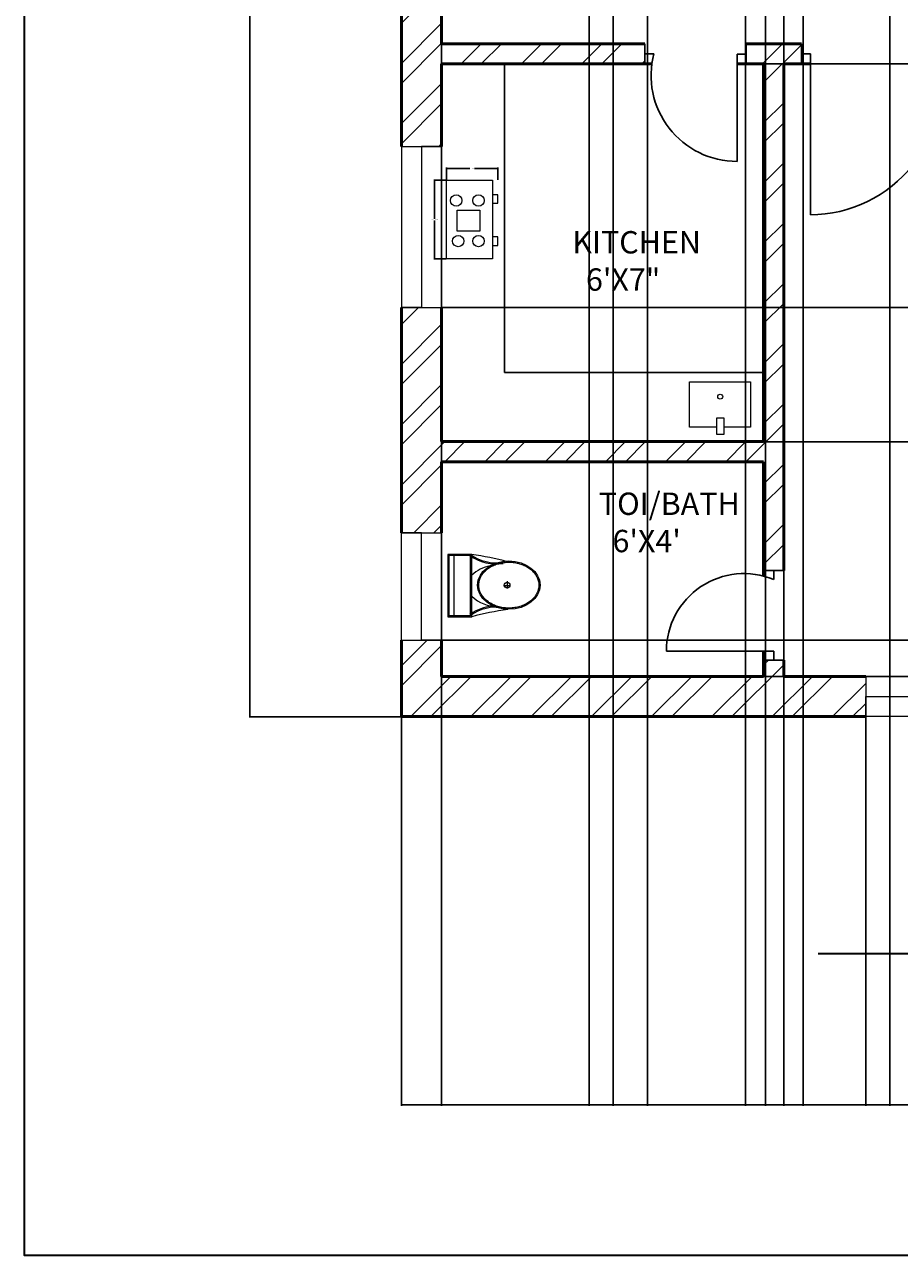
# Model space of a CAD drawing. Units: inches. Extents: x 2310 to 2937, y 1113 to 2410.
# Tile 1 of 23: x 2310 to 2506, y 1616 to 1891. Entities that reach past the tile are written whole.
import ezdxf

# ---------------------------------------------------------------- set-up
doc = ezdxf.new("R2010")
doc.units = ezdxf.units.IN
for name, color, linetype, lineweight in [('A-ANNO-DIMS', 2, 'Continuous', 18), ('A-ANNO-TTLB', 7, 'Continuous', 35), ('A-AREA-IDEN', 7, 'Continuous', 18), ('A-DOOR', 31, 'Continuous', 25), ('A-EQPM', 8, 'Continuous', 18), ('A-FLOR-CASE', 7, 'Continuous', 25), ('A-FLOR-FIXT', 9, 'Continuous', 18), ('A-GLAZ', 191, 'Continuous', 20), ('A-WALL', 7, 'Continuous', 50), ('A-WALL-PATT', 85, 'Continuous', 13)]:
    doc.layers.add(name, color=color, linetype=linetype, lineweight=lineweight)
doc.styles.get("Standard").update_dxf_attribs({"font": 'arial.ttf'})
doc.dimstyles.get("Standard").update_dxf_attribs({"dimtxt": 0.18, "dimasz": 0.18, "dimexe": 0.18, "dimexo": 0.0625, "dimgap": 0.09, "dimtad": 0, "dimtih": 1, "dimtoh": 1, "dimdec": 4, "dimzin": 0, "dimdsep": 46, "dimtxsty": 'Standard', "dimcen": 0.09, "dimadec": 0, "dimazin": 0, "dimtfac": 1, "dimtdec": 4, "dimtofl": 0, "dimtmove": 0, "dimatfit": 3, "dimfxl": 1, "dimtolj": 1, "dimtzin": 0, "dimarcsym": 0})

# ---------------------------------------------------------------- blocks, each defined once
blk = doc.blocks.new('A$C31115884')
for p, q in [((258, 466), (258, 523)), ((283, 498), (223, 498)), ((0, 200), (0, 0)), ((520, 200), (0, 200)), ((10, 190), (10, 10)), ((510, 190), (10, 190)), ((510, 10), (510, 190)), ((520, 0), (520, 200)), ((510, 54), (0, 54)), ((10, 10), (510, 10)), ((0, 0), (520, 0))]:
    blk.add_line(p, q)
blk.add_circle((256, 496), 23.6)
for centre, radius, start, end in [((2778, -205), 2807, 165.4549, 171.7133), ((-295, 403), 365, 324.2091, 9.3499), ((-295, 403), 375, 324.2091, 9.3499), ((139, 406), 293, 315.8436, 2.6563), ((806, 403), 365, 170.6501, 215.7909), ((3237, 905), 2807, 188.2867, 194.5451), ((384, 406), 293, 190.2774, 224.1564), ((806, 403), 375, 179.2036, 215.7909)]:
    blk.add_arc(centre, radius, start, end)
blk.add_ellipse((256, 510), major_axis=(0, -261), ratio=0.772727)
blk.add_open_spline([(256, 259), (263, 259), (270, 260), (288, 262), (299, 265), (320, 273), (330, 278), (350, 291), (360, 299), (378, 316), (386, 326), (402, 347), (409, 358), (421, 383), (427, 395), (436, 422), (440, 436), (445, 465), (447, 480), (448, 509), (448, 524), (445, 553), (443, 568), (436, 596), (432, 610), (422, 636), (416, 649), (402, 672), (395, 683), (379, 703), (370, 712), (351, 728), (341, 735), (321, 746), (310, 751), (289, 757), (278, 759), (256, 761), (245, 761), (223, 757), (212, 754), (191, 746), (181, 741), (161, 728), (151, 720), (133, 703), (125, 693), (110, 672), (103, 660), (90, 636), (85, 623), (76, 596), (72, 582), (67, 553), (66, 538), (64, 509), (65, 494), (68, 465), (70, 450), (77, 422), (81, 408), (91, 382), (97, 370), (111, 346), (118, 335), (135, 316), (144, 307), (162, 291), (172, 284), (193, 273), (203, 269), (225, 262), (236, 260), (250, 259), (253, 259), (256, 259)], degree=3, knots=[0, 0, 0, 0, 0.110105, 0.110105, 0.285049, 0.285049, 0.459994, 0.459994, 0.634938, 0.634938, 0.809882, 0.809882, 0.984827, 0.984827, 1.159771, 1.159771, 1.334715, 1.334715, 1.50966, 1.50966, 1.684604, 1.684604, 1.859549, 1.859549, 2.034493, 2.034493, 2.209437, 2.209437, 2.384382, 2.384382, 2.559326, 2.559326, 2.73427, 2.73427, 2.909215, 2.909215, 3.084159, 3.084159, 3.259103, 3.259103, 3.434048, 3.434048, 3.608992, 3.608992, 3.783936, 3.783936, 3.958881, 3.958881, 4.133825, 4.133825, 4.30877, 4.30877, 4.483714, 4.483714, 4.658658, 4.658658, 4.833603, 4.833603, 5.008547, 5.008547, 5.183491, 5.183491, 5.358436, 5.358436, 5.53338, 5.53338, 5.708324, 5.708324, 5.883269, 5.883269, 6.058213, 6.058213, 6.233158, 6.233158, 6.283185, 6.283185, 6.283185, 6.283185])
blk = doc.blocks.new('SINK-KITCHEN')
blk.add_lwpolyline([(6.01, 11.79), (7.56, 11.79), (7.56, 8.11), (6.01, 8.11)], close=True)
blk.add_lwpolyline([(7.56, 10.17), (13.64, 10.17), (13.64, 0), (0, 0), (0, 10.17), (6.01, 10.17)])
blk.add_circle((6.79, 3.34), 0.556)
blk = doc.blocks.new('RANGE-4-BURNER')
for points in [[(1.2, 17.61), (1.2, 17.61), (1.2, 17.61), (1.2, 17.61)], [(1.2, 17.61), (11.5, 17.61), (11.5, 0), (1.2, 0)], [(1.2, 14.58), (0, 14.58), (0, 12.67), (1.2, 12.67)], [(4.01, 11.43), (9.13, 11.43), (9.13, 6.73), (4.01, 6.73)], [(1.2, 5.14), (0, 5.14), (0, 3.24), (1.2, 3.24)]]:
    blk.add_lwpolyline(points, close=True)
for centre in [(4.34, 13.6), (8.87, 13.6), (4.34, 4.53), (9.32, 4.53)]:
    blk.add_circle(centre, 1.27)
blk = doc.blocks.new('WIN-24IN')
for p, q in [((0, 24), (9, 24)), ((0, 24), (0, 0)), ((9, 24), (4.5, 24)), ((4.5, 24), (4.5, 0)), ((9, 24), (9, 0)), ((4.5, 0), (0, 0)), ((0, 0), (9, 0))]:
    blk.add_line(p, q)
blk = doc.blocks.new('WIN-60IN')
for p, q in [((4.5, 60), (0, 60)), ((0, 60), (9, 60)), ((0, 60), (0, 0)), ((4.5, 0), (4.5, 60)), ((9, 60), (9, 0)), ((0, 0), (9, 0)), ((9, 0), (4.5, 0))]:
    blk.add_line(p, q)
blk = doc.blocks.new('*D25')
at = {"layer": 'A-ANNO-DIMS', "color": 0, "lineweight": -2, "transparency": 16777216}
for p, q in [((2404.5, 1856.48), (2401.74, 1856.48)), ((2401.92, 1856.3), (2401.92, 1847.86)), ((2401.92, 1839.05), (2401.92, 1847.49)), ((2404.5, 1838.87), (2401.74, 1838.87))]:
    blk.add_line(p, q, dxfattribs=at)
at = {"layer": 'A-ANNO-DIMS', "color": 0, "transparency": 16777216}
for points in [[(2401.89, 1856.3), (2401.95, 1856.3), (2401.92, 1856.48)], [(2401.89, 1839.05), (2401.95, 1839.05), (2401.92, 1838.87)]]:
    blk.add_solid(points, dxfattribs=at)
at = {"layer": 'Defpoints', "color": 0, "transparency": 16777216}
for p in [(2404.57, 1856.48), (2401.92, 1838.87), (2404.57, 1838.87)]:
    blk.add_point(p, dxfattribs=at)
at = {"layer": 'A-ANNO-DIMS', "color": 0, "transparency": 16777216, "insert": (2401.92, 1847.67), "char_height": 0.18, "attachment_point": 5}
blk.add_mtext('\\A1;RANGE 18 TYP.', dxfattribs=at)
blk = doc.blocks.new('*D26')
at = {"layer": 'A-ANNO-DIMS', "color": 0, "lineweight": -2, "transparency": 16777216}
for p, q in [((2404.57, 1856.54), (2404.57, 1859.3)), ((2404.75, 1859.12), (2409.8, 1859.12)), ((2415.89, 1859.12), (2410.84, 1859.12)), ((2416.07, 1856.54), (2416.07, 1859.3))]:
    blk.add_line(p, q, dxfattribs=at)
at = {"layer": 'A-ANNO-DIMS', "color": 0, "transparency": 16777216}
for points in [[(2404.75, 1859.15), (2404.75, 1859.09), (2404.57, 1859.12)], [(2415.89, 1859.15), (2415.89, 1859.09), (2416.07, 1859.12)]]:
    blk.add_solid(points, dxfattribs=at)
at = {"layer": 'Defpoints', "color": 0, "transparency": 16777216}
for p in [(2404.57, 1859.12), (2404.57, 1856.48), (2416.07, 1856.48)]:
    blk.add_point(p, dxfattribs=at)
at = {"layer": 'A-ANNO-DIMS', "color": 0, "transparency": 16777216, "insert": (2410.32, 1859.12), "char_height": 0.18, "attachment_point": 5}
blk.add_mtext('\\A1;12 TYP.', dxfattribs=at)
blk = doc.blocks.new('*D40')
at = {"layer": 'A-ANNO-DIMS', "color": 0, "lineweight": -2, "transparency": 16777216}
for p, q in [((2394.42, 2356.51), (2360.46, 2356.51)), ((2360.64, 2356.33), (2360.64, 2046.7)), ((2360.64, 1736.69), (2360.64, 2046.33)), ((2394.42, 1736.51), (2360.46, 1736.51))]:
    blk.add_line(p, q, dxfattribs=at)
at = {"layer": 'A-ANNO-DIMS', "color": 0, "transparency": 16777216}
for points in [[(2360.61, 2356.33), (2360.67, 2356.33), (2360.64, 2356.51)], [(2360.61, 1736.69), (2360.67, 1736.69), (2360.64, 1736.51)]]:
    blk.add_solid(points, dxfattribs=at)
at = {"layer": 'Defpoints', "color": 0, "transparency": 16777216}
for p in [(2360.64, 2356.51), (2394.49, 2356.51), (2394.49, 1736.51)]:
    blk.add_point(p, dxfattribs=at)
at = {"layer": 'A-ANNO-DIMS', "color": 0, "transparency": 16777216, "insert": (2360.64, 2046.51), "char_height": 0.18, "attachment_point": 5}
blk.add_mtext('\\A1;620', dxfattribs=at)
blk = doc.blocks.new('*D41')
at = {"layer": 'A-ANNO-DIMS', "color": 0, "lineweight": -2, "transparency": 16777216}
for p, q in [((2479.99, 2347.45), (2479.99, 1649.5)), ((2503.66, 2347.45), (2503.66, 1649.5)), ((2480.17, 1649.68), (2491.36, 1649.68)), ((2503.48, 1649.68), (2492.29, 1649.68))]:
    blk.add_line(p, q, dxfattribs=at)
at = {"layer": 'A-ANNO-DIMS', "color": 0, "transparency": 16777216}
for points in [[(2480.17, 1649.71), (2480.17, 1649.65), (2479.99, 1649.68)], [(2503.48, 1649.71), (2503.48, 1649.65), (2503.66, 1649.68)]]:
    blk.add_solid(points, dxfattribs=at)
at = {"layer": 'Defpoints', "color": 0, "transparency": 16777216}
for p in [(2479.99, 2347.51), (2503.66, 2347.51), (2503.66, 1649.68)]:
    blk.add_point(p, dxfattribs=at)
at = {"layer": 'A-ANNO-DIMS', "color": 0, "transparency": 16777216, "insert": (2491.82, 1649.68), "char_height": 0.18, "attachment_point": 5}
blk.add_mtext('\\A1;23.676', dxfattribs=at)
blk = doc.blocks.new('*D43')
at = {"layer": 'A-ANNO-DIMS', "color": 0, "lineweight": -2, "transparency": 16777216}
for p, q in [((2394.49, 1736.45), (2394.49, 1649.5)), ((2498.31, 1736.45), (2498.31, 1649.5)), ((2394.67, 1649.68), (2445.94, 1649.68)), ((2498.13, 1649.68), (2446.85, 1649.68))]:
    blk.add_line(p, q, dxfattribs=at)
at = {"layer": 'A-ANNO-DIMS', "color": 0, "transparency": 16777216}
for points in [[(2394.67, 1649.71), (2394.67, 1649.65), (2394.49, 1649.68)], [(2498.13, 1649.71), (2498.13, 1649.65), (2498.31, 1649.68)]]:
    blk.add_solid(points, dxfattribs=at)
at = {"layer": 'Defpoints', "color": 0, "transparency": 16777216}
for p in [(2394.49, 1736.51), (2498.31, 1736.51), (2498.31, 1649.68)]:
    blk.add_point(p, dxfattribs=at)
at = {"layer": 'A-ANNO-DIMS', "color": 0, "transparency": 16777216, "insert": (2446.4, 1649.68), "char_height": 0.18, "attachment_point": 5}
blk.add_mtext('\\A1;103.82', dxfattribs=at)
blk = doc.blocks.new('*D55')
at = {"layer": 'A-ANNO-DIMS', "color": 0, "lineweight": -2, "transparency": 16777216}
for p, q in [((2403.55, 1753.64), (2858.02, 1753.64)), ((2857.84, 1753.46), (2857.84, 1749.76)), ((2857.84, 1745.69), (2857.84, 1749.4)), ((2403.55, 1745.51), (2858.02, 1745.51))]:
    blk.add_line(p, q, dxfattribs=at)
at = {"layer": 'A-ANNO-DIMS', "color": 0, "transparency": 16777216}
for points in [[(2857.81, 1753.46), (2857.87, 1753.46), (2857.84, 1753.64)], [(2857.81, 1745.69), (2857.87, 1745.69), (2857.84, 1745.51)]]:
    blk.add_solid(points, dxfattribs=at)
at = {"layer": 'Defpoints', "color": 0, "transparency": 16777216}
for p in [(2403.49, 1753.64), (2857.84, 1753.64), (2403.49, 1745.51)]:
    blk.add_point(p, dxfattribs=at)
at = {"layer": 'A-ANNO-DIMS', "color": 0, "transparency": 16777216, "insert": (2857.84, 1749.58), "char_height": 0.18, "attachment_point": 5}
blk.add_mtext('\\A1;8.127', dxfattribs=at)
blk = doc.blocks.new('*D56')
at = {"layer": 'A-ANNO-DIMS', "color": 0, "lineweight": -2, "transparency": 16777216}
for p, q in [((2403.55, 1828.04), (2858.02, 1828.04)), ((2857.84, 1827.86), (2857.84, 1813.21)), ((2857.84, 1798.19), (2857.84, 1812.85)), ((2403.55, 1798.01), (2858.02, 1798.01))]:
    blk.add_line(p, q, dxfattribs=at)
at = {"layer": 'A-ANNO-DIMS', "color": 0, "transparency": 16777216}
for points in [[(2857.81, 1827.86), (2857.87, 1827.86), (2857.84, 1828.04)], [(2857.81, 1798.19), (2857.87, 1798.19), (2857.84, 1798.01)]]:
    blk.add_solid(points, dxfattribs=at)
at = {"layer": 'Defpoints', "color": 0, "transparency": 16777216}
for p in [(2403.49, 1828.04), (2857.84, 1828.04), (2403.49, 1798.01)]:
    blk.add_point(p, dxfattribs=at)
at = {"layer": 'A-ANNO-DIMS', "color": 0, "transparency": 16777216, "insert": (2857.84, 1813.03), "char_height": 0.18, "attachment_point": 5}
blk.add_mtext('\\A1;30.03', dxfattribs=at)
blk = doc.blocks.new('*D58')
at = {"layer": 'A-ANNO-DIMS', "color": 0, "lineweight": -2, "transparency": 16777216}
for p, q in [((2475.55, 1882.51), (2858.02, 1882.51)), ((2857.84, 1882.33), (2857.84, 1840.45)), ((2857.84, 1798.19), (2857.84, 1840.08)), ((2475.55, 1798.01), (2858.02, 1798.01))]:
    blk.add_line(p, q, dxfattribs=at)
at = {"layer": 'A-ANNO-DIMS', "color": 0, "transparency": 16777216}
for points in [[(2857.81, 1882.33), (2857.87, 1882.33), (2857.84, 1882.51)], [(2857.81, 1798.19), (2857.87, 1798.19), (2857.84, 1798.01)]]:
    blk.add_solid(points, dxfattribs=at)
at = {"layer": 'Defpoints', "color": 0, "transparency": 16777216}
for p in [(2475.49, 1882.51), (2857.84, 1882.51), (2475.49, 1798.01)]:
    blk.add_point(p, dxfattribs=at)
at = {"layer": 'A-ANNO-DIMS', "color": 0, "transparency": 16777216, "insert": (2857.84, 1840.26), "char_height": 0.18, "attachment_point": 5}
blk.add_mtext('\\A1;84.5', dxfattribs=at)
blk = doc.blocks.new('*D60')
at = {"layer": 'A-ANNO-DIMS', "color": 0, "lineweight": -2, "transparency": 16777216}
for p, q in [((2449.5, 2205.95), (2449.5, 1649.5)), ((2471.44, 2205.95), (2471.44, 1649.5)), ((2449.68, 1649.68), (2460.01, 1649.68)), ((2471.26, 1649.68), (2460.94, 1649.68))]:
    blk.add_line(p, q, dxfattribs=at)
at = {"layer": 'A-ANNO-DIMS', "color": 0, "transparency": 16777216}
for points in [[(2449.68, 1649.71), (2449.68, 1649.65), (2449.5, 1649.68)], [(2471.26, 1649.71), (2471.26, 1649.65), (2471.44, 1649.68)]]:
    blk.add_solid(points, dxfattribs=at)
at = {"layer": 'Defpoints', "color": 0, "transparency": 16777216}
for p in [(2449.5, 2206.01), (2471.44, 2206.01), (2471.44, 1649.68)]:
    blk.add_point(p, dxfattribs=at)
at = {"layer": 'A-ANNO-DIMS', "color": 0, "transparency": 16777216, "insert": (2460.47, 1649.68), "char_height": 0.18, "attachment_point": 5}
blk.add_mtext('\\A1;21.936', dxfattribs=at)
blk = doc.blocks.new('*D61')
at = {"layer": 'A-ANNO-DIMS', "color": 0, "lineweight": -2, "transparency": 16777216}
for p, q in [((2484.33, 2205.95), (2484.33, 1649.5)), ((2514.27, 2205.95), (2514.27, 1649.5)), ((2484.51, 1649.68), (2498.9, 1649.68)), ((2514.09, 1649.68), (2499.69, 1649.68))]:
    blk.add_line(p, q, dxfattribs=at)
at = {"layer": 'A-ANNO-DIMS', "color": 0, "transparency": 16777216}
for points in [[(2484.51, 1649.71), (2484.51, 1649.65), (2484.33, 1649.68)], [(2514.09, 1649.71), (2514.09, 1649.65), (2514.27, 1649.68)]]:
    blk.add_solid(points, dxfattribs=at)
at = {"layer": 'Defpoints', "color": 0, "transparency": 16777216}
for p in [(2484.33, 2206.01), (2514.27, 2206.01), (2514.27, 1649.68)]:
    blk.add_point(p, dxfattribs=at)
at = {"layer": 'A-ANNO-DIMS', "color": 0, "transparency": 16777216, "insert": (2499.3, 1649.68), "char_height": 0.18, "attachment_point": 5}
blk.add_mtext('\\A1;29.94', dxfattribs=at)
blk = doc.blocks.new('*D63')
at = {"layer": 'A-ANNO-DIMS', "color": 0, "lineweight": -2, "transparency": 16777216}
for p, q in [((2436.46, 1999.45), (2436.46, 1649.5)), ((2524.46, 1999.45), (2524.46, 1649.5)), ((2436.64, 1649.68), (2480.25, 1649.68)), ((2524.28, 1649.68), (2480.68, 1649.68))]:
    blk.add_line(p, q, dxfattribs=at)
at = {"layer": 'A-ANNO-DIMS', "color": 0, "transparency": 16777216}
for points in [[(2436.64, 1649.71), (2436.64, 1649.65), (2436.46, 1649.68)], [(2524.28, 1649.71), (2524.28, 1649.65), (2524.46, 1649.68)]]:
    blk.add_solid(points, dxfattribs=at)
at = {"layer": 'Defpoints', "color": 0, "transparency": 16777216}
for p in [(2436.46, 1999.51), (2524.46, 1999.51), (2524.46, 1649.68)]:
    blk.add_point(p, dxfattribs=at)
at = {"layer": 'A-ANNO-DIMS', "color": 0, "transparency": 16777216, "insert": (2480.46, 1649.68), "char_height": 0.18, "attachment_point": 5}
blk.add_mtext('\\A1;88', dxfattribs=at)
blk = doc.blocks.new('*D65')
at = {"layer": 'A-ANNO-DIMS', "color": 0, "lineweight": -2, "transparency": 16777216}
for p, q in [((2403.49, 2093.45), (2403.49, 1649.5)), ((2436.46, 2093.45), (2436.46, 1649.5)), ((2403.67, 1649.68), (2419.58, 1649.68)), ((2436.28, 1649.68), (2420.37, 1649.68))]:
    blk.add_line(p, q, dxfattribs=at)
at = {"layer": 'A-ANNO-DIMS', "color": 0, "transparency": 16777216}
for points in [[(2403.67, 1649.71), (2403.67, 1649.65), (2403.49, 1649.68)], [(2436.28, 1649.71), (2436.28, 1649.65), (2436.46, 1649.68)]]:
    blk.add_solid(points, dxfattribs=at)
at = {"layer": 'Defpoints', "color": 0, "transparency": 16777216}
for p in [(2403.49, 2093.51), (2436.46, 2093.51), (2436.46, 1649.68)]:
    blk.add_point(p, dxfattribs=at)
at = {"layer": 'A-ANNO-DIMS', "color": 0, "transparency": 16777216, "insert": (2419.98, 1649.68), "char_height": 0.18, "attachment_point": 5}
blk.add_mtext('\\A1;32.98', dxfattribs=at)
blk = doc.blocks.new('*D69')
at = {"layer": 'A-ANNO-DIMS', "color": 0, "lineweight": -2, "transparency": 16777216}
for p, q in [((2441.86, 2131.96), (2441.86, 1649.5)), ((2475.89, 2131.96), (2475.89, 1649.5)), ((2442.04, 1649.68), (2458.48, 1649.68)), ((2475.71, 1649.68), (2459.27, 1649.68))]:
    blk.add_line(p, q, dxfattribs=at)
at = {"layer": 'A-ANNO-DIMS', "color": 0, "transparency": 16777216}
for points in [[(2442.04, 1649.71), (2442.04, 1649.65), (2441.86, 1649.68)], [(2475.71, 1649.71), (2475.71, 1649.65), (2475.89, 1649.68)]]:
    blk.add_solid(points, dxfattribs=at)
at = {"layer": 'Defpoints', "color": 0, "transparency": 16777216}
for p in [(2441.86, 2132.02), (2475.89, 2132.02), (2475.89, 1649.68)]:
    blk.add_point(p, dxfattribs=at)
at = {"layer": 'A-ANNO-DIMS', "color": 0, "transparency": 16777216, "insert": (2458.88, 1649.68), "char_height": 0.18, "attachment_point": 5}
blk.add_mtext('\\A1;34.03', dxfattribs=at)

msp = doc.modelspace()

# ---------------------------------------------------------------- hatches: boundary and pattern name
at = {"layer": 'A-WALL-PATT'}
h = msp.add_hatch(dxfattribs=at)
h.set_pattern_fill('ANSI32', color=256)
h.paths.add_polyline_path([(2639.1394, 2356.5139), (2563.662, 2356.5139), (2563.662, 2347.5139), (2606.9859, 2347.5139), (2606.9859, 2210.5139), (2514.2692, 2210.5139), (2514.2692, 2206.0139), (2606.9859, 2206.0139), (2606.9859, 2098.0139), (2602.689, 2098.0139), (2602.689, 2093.5139), (2615.5262, 2093.5139), (2615.5262, 2095.7639), (2615.5262, 2098.0139), (2611.4859, 2098.0139), (2611.4859, 2206.0139), (2703.9391, 2206.0139), (2703.9391, 2208.2639), (2703.9391, 2210.5139), (2611.4859, 2210.5139), (2611.4859, 2347.5139), (2639.1394, 2347.5139)])
h.paths.add_polyline_path([(2823.9859, 2356.5139), (2699.1394, 2356.5139), (2699.1394, 2347.5139), (2738.4859, 2347.5139), (2738.4859, 2343.9266), (2742.9859, 2343.9266), (2742.9859, 2347.5139), (2814.9859, 2347.5139), (2814.9859, 2336.76), (2823.9859, 2336.76)])
h.paths.add_polyline_path([(2823.9859, 2312.76), (2814.9859, 2312.76), (2814.9859, 2299.5139), (2742.9859, 2299.5139), (2742.9859, 2323.0159), (2740.7359, 2323.0159), (2738.4859, 2323.0159), (2738.4859, 2210.5139), (2734.5483, 2210.5139), (2734.5483, 2206.0139), (2746.8769, 2206.0139), (2746.8769, 2208.2639), (2746.8769, 2210.5139), (2742.9859, 2210.5139), (2742.9859, 2295.0139), (2814.9859, 2295.0139), (2814.9859, 2269.8977), (2823.9859, 2269.8977)])
h.paths.add_polyline_path([(2823.9859, 2210.5139), (2823.9859, 2233.8977), (2819.4859, 2233.8977), (2814.9859, 2233.8977), (2814.9859, 2210.5139), (2769.9745, 2210.5139), (2769.9745, 2206.0139), (2814.9859, 2206.0139), (2814.9859, 2178.3027), (2823.9859, 2178.3027)])
h.paths.add_polyline_path([(2823.9859, 2118.3027), (2819.4859, 2118.3027), (2814.9859, 2118.3027), (2814.9859, 2098.0139), (2647.0333, 2098.0139), (2647.0333, 2093.5139), (2814.9859, 2093.5139), (2814.9859, 1999.5139), (2650.6052, 1999.5139), (2650.6052, 1995.0139), (2814.9859, 1995.0139), (2814.9859, 1969.9784), (2823.9859, 1969.9784)])
h.paths.add_polyline_path([(2403.4859, 2093.5139), (2569.9888, 2093.5139), (2569.9888, 2095.7639), (2569.9888, 2098.0139), (2403.4859, 2098.0139), (2403.4859, 2131.7587), (2394.4859, 2131.7587), (2394.4859, 1967.522), (2403.4859, 1967.522), (2403.4859, 1995.0139), (2569.8903, 1995.0139), (2569.8903, 1997.2639), (2569.8903, 1999.5139), (2403.4859, 1999.5139)])
h.paths.add_polyline_path([(2503.662, 2356.5139), (2394.4859, 2356.5139), (2394.4859, 2337.9231), (2398.9859, 2337.9231), (2403.4859, 2337.9231), (2403.4859, 2347.5139), (2475.4859, 2347.5139), (2475.4859, 2343.0384), (2479.9859, 2343.0384), (2479.9859, 2347.5139), (2503.662, 2347.5139)])
h.paths.add_polyline_path([(2498.3065, 1745.5139), (2479.9859, 1745.5139), (2479.9859, 1749.1663), (2477.7359, 1749.1663), (2475.4859, 1749.1663), (2475.4859, 1745.5139), (2403.4859, 1745.5139), (2403.4859, 1753.6409), (2398.9859, 1753.6409), (2394.4859, 1753.6409), (2394.4859, 1736.5139), (2498.3065, 1736.5139), (2498.3065, 1741.0139)])
h.paths.add_polyline_path([(2479.9859, 1882.5139), (2483.9367, 1882.5139), (2483.9367, 1887.0139), (2471.5501, 1887.0139), (2471.5501, 1885.1969), (2471.5501, 1882.5139), (2475.4859, 1882.5139), (2475.4859, 1798.0139), (2403.4859, 1798.0139), (2403.4859, 1828.0433), (2402.2852, 1828.0433), (2394.4859, 1828.0433), (2394.4859, 1777.6409), (2403.4859, 1777.6409), (2403.4859, 1793.5139), (2475.4859, 1793.5139), (2475.4859, 1769.1696), (2479.9859, 1769.1696)])
h.paths.add_polyline_path([(2403.4859, 1907.522), (2398.9859, 1907.522), (2394.4859, 1907.522), (2394.4859, 1864.0433), (2403.4859, 1864.0433), (2403.4859, 1882.5139), (2448.9325, 1882.5139), (2448.9325, 1884.7639), (2448.9325, 1887.0139), (2403.4859, 1887.0139)])
h.paths.add_polyline_path([(2702.2061, 1887.0139), (2611.4859, 1887.0139), (2611.4859, 1995.0139), (2615.6132, 1995.0139), (2615.6132, 1999.5139), (2602.4798, 1999.5139), (2602.4798, 1997.2639), (2602.4798, 1995.0139), (2606.9859, 1995.0139), (2606.9859, 1887.0139), (2516.2443, 1887.0139), (2516.2443, 1884.7639), (2516.2443, 1882.5139), (2606.9859, 1882.5139), (2606.9859, 1745.5139), (2558.3065, 1745.5139), (2558.3065, 1736.5139), (2638.8921, 1736.5139), (2638.8921, 1741.0139), (2638.8921, 1745.5139), (2611.4859, 1745.5139), (2611.4859, 1882.5139), (2702.2061, 1882.5139)])
h.paths.add_polyline_path([(2823.9859, 1909.9784), (2819.4859, 1909.9784), (2814.9859, 1909.9784), (2814.9859, 1887.0139), (2769.144, 1887.0139), (2769.144, 1884.7639), (2769.144, 1882.5139), (2814.9859, 1882.5139), (2814.9859, 1854.1704), (2823.9859, 1854.1704)])
h.paths.add_polyline_path([(2823.9859, 1818.1704), (2819.4859, 1818.1704), (2814.9859, 1818.1704), (2814.9859, 1798.0139), (2742.9859, 1798.0139), (2742.9859, 1882.5139), (2746.805, 1882.5139), (2746.805, 1887.0139), (2733.7334, 1887.0139), (2733.7334, 1884.7639), (2733.7334, 1882.5139), (2738.4859, 1882.5139), (2738.4859, 1771.1728), (2740.7359, 1771.1728), (2742.9859, 1771.1728), (2742.9859, 1793.5139), (2814.9859, 1793.5139), (2814.9859, 1783.6684), (2823.9859, 1783.6684)])
h.paths.add_polyline_path([(2823.9859, 1759.6684), (2814.9859, 1759.6684), (2814.9859, 1745.5139), (2742.9859, 1745.5139), (2742.9859, 1748.9831), (2740.7359, 1748.9831), (2738.4859, 1748.9831), (2738.4859, 1745.5139), (2698.8921, 1745.5139), (2698.8921, 1736.5139), (2823.9859, 1736.5139)])

# ---------------------------------------------------------------- linework, layer by layer
at = {"layer": 'A-ANNO-TTLB'}
msp.add_line((2487.6418, 1683.5307), (2761.8399, 1683.5307), dxfattribs=at)
msp.add_lwpolyline([(2310.2498, 2409.8427), (2937.0534, 2409.8427), (2937.0534, 1616.036), (2310.2498, 1616.036)], close=True, dxfattribs=at)
at = {"layer": 'A-DOOR'}
for p, q in [((2448.9325, 1887.0139), (2448.9325, 1882.5139)), ((2471.5501, 1887.0139), (2471.5501, 1885.1969)), ((2483.9367, 1882.5139), (2483.9367, 1887.0139)), ((2483.9367, 1887.0139), (2483.9367, 1884.7639)), ((2448.9325, 1882.5139), (2448.9325, 1884.7639)), ((2448.9325, 1884.7639), (2450.9325, 1884.7639)), ((2471.5501, 1884.6742), (2469.5501, 1884.6742)), ((2469.5501, 1884.6742), (2469.5501, 1860.6742)), ((2471.5501, 1885.1969), (2471.5501, 1882.5139)), ((2471.5501, 1882.5139), (2471.5501, 1884.6742)), ((2483.9367, 1884.7639), (2485.9367, 1884.7639)), ((2485.9367, 1884.7639), (2485.9367, 1848.7639)), ((2475.4859, 1769.1696), (2479.9859, 1769.1696)), ((2479.9859, 1769.1696), (2477.7359, 1769.1696)), ((2477.7359, 1769.1696), (2477.7359, 1767.1696)), ((2477.7359, 1751.1663), (2453.7359, 1751.1663)), ((2477.7359, 1749.1663), (2477.7359, 1751.1663)), ((2475.4859, 1749.1663), (2479.9859, 1749.1663)), ((2479.9859, 1749.1663), (2477.7359, 1749.1663))]:
    msp.add_line(p, q, dxfattribs=at)
for centre, radius, start, end in [((2469.5501, 1879.9133), 19.2391, 165.396712, 270), ((2485.9367, 1877.8934), 29.1295, 270, 13.642354), ((2471.0715, 1751.1663), 17.3355, 67.39102, 180)]:
    msp.add_arc(centre, radius, start, end, dxfattribs=at)
at = {"layer": 'A-FLOR-CASE'}
for p, q in [((2417.5784, 1882.5139), (2417.5784, 1882.5139)), ((2417.5784, 1882.5139), (2417.5784, 1813.4436)), ((2417.5784, 1813.4436), (2475.4859, 1813.4436))]:
    msp.add_line(p, q, dxfattribs=at)
at = {"layer": 'A-GLAZ'}
for p, q in [((2394.4859, 1864.0433), (2403.4859, 1864.0433)), ((2394.4859, 1864.0433), (2394.4859, 1828.0433)), ((2403.4859, 1864.0433), (2398.9859, 1864.0433)), ((2398.9859, 1864.0433), (2398.9859, 1828.0433)), ((2403.4859, 1864.0433), (2403.4859, 1828.0433)), ((2398.9859, 1828.0433), (2394.4859, 1828.0433)), ((2394.4859, 1828.0433), (2402.2852, 1828.0433)), ((2402.2852, 1828.0433), (2403.4859, 1828.0433)), ((2498.3065, 1745.5139), (2498.3065, 1745.5139))]:
    msp.add_line(p, q, dxfattribs=at)
at = {"layer": 'A-WALL'}
for p, q in [((2394.4859, 1907.522), (2394.4859, 1864.0433)), ((2403.4859, 1907.522), (2403.4859, 1887.0139)), ((2403.4859, 1887.0139), (2448.9325, 1887.0139)), ((2471.5501, 1887.0139), (2483.9367, 1887.0139)), ((2403.4859, 1882.5139), (2450.4876, 1882.5139)), ((2403.4859, 1882.5139), (2403.4859, 1864.0433)), ((2469.5501, 1882.5139), (2475.4859, 1882.5139)), ((2475.4859, 1882.5139), (2475.4859, 1798.0139)), ((2479.9859, 1882.5139), (2479.9859, 1769.1696)), ((2479.9859, 1882.5139), (2485.9367, 1882.5139)), ((2394.4859, 1828.0433), (2394.4859, 1777.6409)), ((2403.4859, 1828.0433), (2403.4859, 1798.0139)), ((2403.4859, 1798.0139), (2475.4859, 1798.0139)), ((2403.4859, 1793.5139), (2475.4859, 1793.5139)), ((2403.4859, 1793.5139), (2403.4859, 1777.6409)), ((2475.4859, 1793.5139), (2475.4859, 1767.9304)), ((2394.4859, 1753.6409), (2394.4859, 1736.5139)), ((2403.4859, 1753.6409), (2403.4859, 1745.5139)), ((2475.4859, 1751.1663), (2475.4859, 1745.5139)), ((2479.9859, 1749.1663), (2479.9859, 1745.5139)), ((2403.4859, 1745.5139), (2475.4859, 1745.5139)), ((2479.9859, 1745.5139), (2498.3065, 1745.5139)), ((2394.4859, 1736.5139), (2498.3065, 1736.5139))]:
    msp.add_line(p, q, dxfattribs=at)

# ---------------------------------------------------------------- block references
at = {"layer": 'A-EQPM', "rotation": 180}
msp.add_blockref('RANGE-4-BURNER', (2416.0658, 1856.4793), dxfattribs=at)
at = {"layer": 'A-FLOR-FIXT', "rotation": 180}
msp.add_blockref('SINK-KITCHEN', (2472.5636, 1811.4144), dxfattribs=at)
at = {"layer": 'A-FLOR-FIXT', "xscale": 0.0268011493576733, "yscale": 0.0268011493576733, "zscale": 0.0268011493576733, "rotation": 270}
msp.add_blockref('A$C31115884', (2404.8416, 1772.7938), dxfattribs=at)
at = {"layer": 'A-GLAZ', "extrusion": (0, 0, -1), "zscale": -1, "rotation": 180}
msp.add_blockref('WIN-24IN', (-2394.4859, 1777.6409), dxfattribs=at)
at = {"layer": 'A-GLAZ', "rotation": 270}
msp.add_blockref('WIN-60IN', (2498.3065, 1745.5139), dxfattribs=at)

# ---------------------------------------------------------------- texts
at = {"layer": 'A-AREA-IDEN', "char_height": 5, "attachment_point": 1}
for s, width, insert in [('    KITCHEN\\P      6\'X7"', 249.306514, (2426.5872, 1845.1001)), ("  TOI/BATH\\P    6'X4'", 253.303889, (2435.5765, 1786.6243))]:
    msp.add_mtext_dynamic_manual_height_columns(s, width=width, gutter_width=12.5, heights=[0], dxfattribs=dict(at, insert=insert))

# ---------------------------------------------------------------- dimensions: what is measured, and where the dimension line sits
at = {"layer": 'A-ANNO-DIMS'}
for base, p1, p2, override, picture, middle in [((2360.6359, 2356.5139), (2394.4859, 1736.5139), (2394.4859, 2356.5139), {"dimdec": 0, "dimlfac": 1, "dimrnd": 0, "dimzin": 0, "dimdsep": 46, "dimlunit": 2}, '*D40', (2360.6359, 2046.5139)), ((2857.8359, 1882.5139), (2475.4859, 1798.0139), (2475.4859, 1882.5139), {"dimdec": 1, "dimlfac": 1, "dimrnd": 0, "dimzin": 0, "dimdsep": 46, "dimlunit": 2}, '*D58', (2857.8359, 1840.2639)), ((2857.8359, 1828.0433), (2403.4859, 1798.0139), (2403.4859, 1828.0433), {"dimdec": 2, "dimlfac": 1, "dimrnd": 0, "dimzin": 0, "dimdsep": 46, "dimlunit": 2}, '*D56', (2857.8359, 1813.0286)), ((2857.8359, 1753.6409), (2403.4859, 1745.5139), (2403.4859, 1753.6409), {"dimdec": 3, "dimlfac": 1, "dimrnd": 0, "dimzin": 0, "dimdsep": 46, "dimlunit": 2}, '*D55', (2857.8359, 1749.5774))]:
    dim = msp.add_linear_dim(base=base, p1=p1, p2=p2, angle=90, dimstyle='Standard', override=override, dxfattribs=at)
    dim.commit()
    dim.dimension.update_dxf_attribs({"geometry": picture, "text_midpoint": middle})
for base, p1, p2, override, picture, middle in [((2503.662, 1649.6807), (2479.9859, 2347.5139), (2503.662, 2347.5139), {"dimdec": 3, "dimlfac": 1, "dimrnd": 0, "dimzin": 0, "dimdsep": 46, "dimlunit": 2}, '*D41', (2491.824, 1649.6807)), ((2471.4388, 1649.6807), (2449.5024, 2206.0139), (2471.4388, 2206.0139), {"dimdec": 3, "dimlfac": 1, "dimrnd": 0, "dimzin": 0, "dimdsep": 46, "dimlunit": 2}, '*D60', (2460.4706, 1649.6807)), ((2514.2692, 1649.6807), (2484.3278, 2206.0139), (2514.2692, 2206.0139), {"dimdec": 2, "dimlfac": 1, "dimrnd": 0, "dimzin": 0, "dimdsep": 46, "dimlunit": 2}, '*D61', (2499.2985, 1649.6807)), ((2475.8929, 1649.6807), (2441.8613, 2132.0241), (2475.8929, 2132.0241), {"dimdec": 2, "dimlfac": 1, "dimrnd": 0, "dimzin": 0, "dimdsep": 46, "dimlunit": 2}, '*D69', (2458.8771, 1649.6807)), ((2436.4647, 1649.6807), (2403.4859, 2093.5139), (2436.4647, 2093.5139), {"dimdec": 2, "dimlfac": 1, "dimrnd": 0, "dimzin": 0, "dimdsep": 46, "dimlunit": 2}, '*D65', (2419.9753, 1649.6807)), ((2524.4647, 1649.6807), (2436.4647, 1999.5139), (2524.4647, 1999.5139), {"dimdec": 0, "dimlfac": 1, "dimrnd": 0, "dimzin": 0, "dimdsep": 46, "dimlunit": 2}, '*D63', (2480.4647, 1649.6807)), ((2498.3065, 1649.6807), (2394.4859, 1736.5139), (2498.3065, 1736.5139), {"dimdec": 2, "dimlfac": 1, "dimrnd": 0, "dimzin": 0, "dimdsep": 46, "dimlunit": 2}, '*D43', (2446.3962, 1649.6807))]:
    dim = msp.add_linear_dim(base=base, p1=p1, p2=p2, dimstyle='Standard', override=override, dxfattribs=at)
    dim.commit()
    dim.dimension.update_dxf_attribs({"geometry": picture, "text_midpoint": middle})
for base, p1, p2, angle, text, picture, middle in [((2404.5651, 1859.1207), (2416.0658, 1856.4793), (2404.5651, 1856.4793), 180, '<> TYP.', '*D26', (2410.3155, 1859.1207)), ((2401.9238, 1838.87), (2404.5651, 1856.4793), (2404.5651, 1838.87), 270, 'RANGE <> TYP.', '*D25', (2401.9238, 1847.6747))]:
    dim = msp.add_linear_dim(base=base, p1=p1, p2=p2, angle=angle, text=text, dimstyle='Standard', override={"dimdec": 0, "dimlfac": 1, "dimrnd": 0, "dimzin": 0, "dimdsep": 46, "dimlunit": 2}, dxfattribs=at)
    dim.commit()
    dim.dimension.update_dxf_attribs({"geometry": picture, "text_midpoint": middle})

doc.saveas('drawing.dxf')
